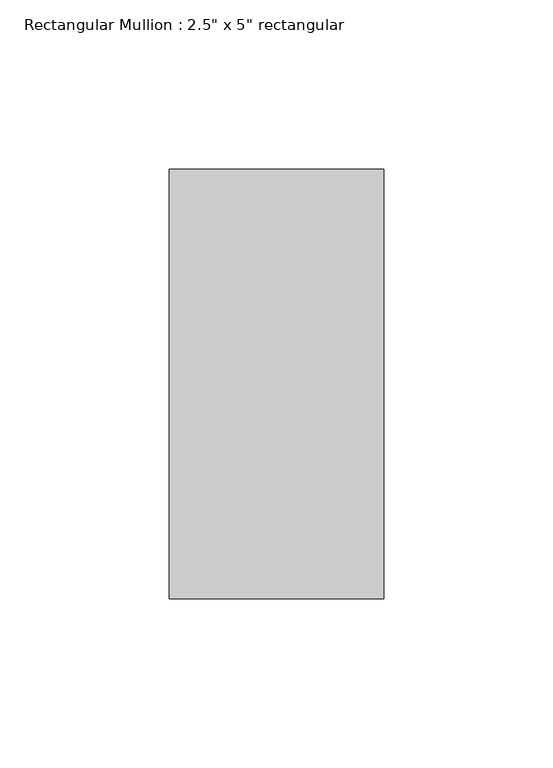
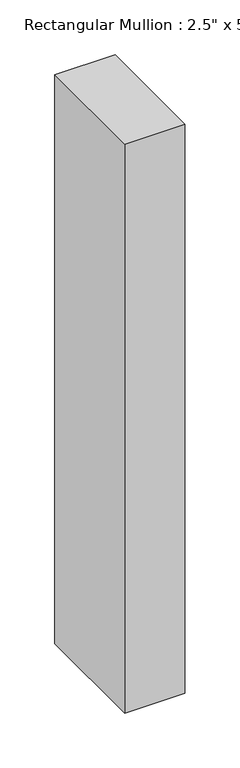
"""IFC4 building model written with IfcOpenShell, lengths in millimetres: member geometry."""

from ifc_helpers import new_model, si_unit, frame, origin, place, context, project, spatial, polyline, outline, extrude, source, transform, mapped, element, save


def member_7f909d8d(model_context):
    return source(origin(), model_context, "Body", "SweptSolid", [
        extrude(outline(polyline([(0.0, 63.5), (0.0, -63.5), (-63.5, -63.5), (-63.5, 63.5), (0.0, 63.5)])), frame((0.0, 0.0, -632.8833333), z_axis=(0.0, 0.0, 1.0), x_axis=(1.0, 0.0, 0.0)), (0.0, 0.0, 1.0), 632.8833333),
    ])


if __name__ == "__main__":
    model = new_model("IFC4")
    model_context = context("Model", 3, world=origin())
    ifc_project = project(units=[si_unit("LENGTHUNIT", "METRE", prefix="MILLI")], contexts=[model_context])
    site = spatial("IfcSite", under=ifc_project)
    building = spatial("IfcBuilding", under=site)
    placement = place(None, origin())
    member_shape = member_7f909d8d(model_context)
    element("IfcMember", 1, ObjectType="Rectangular Mullion : 2.5\" x 5\" rectangular", at=placement, inside=building, context=model_context, shape_type="MappedRepresentation", body=[
        mapped(member_shape, transform((0.0, 0.0, 0.0), x_axis=(1.0, 0.0, 0.0), y_axis=(0.0, 1.0, 0.0), z_axis=(0.0, 0.0, 1.0))),
    ])
    save(model, "model.ifc")

# Revit data of these elements
# Type "Rectangular Mullion : 2.5\" x 5\" rectangular"
#   built-in parameter 1007304 = 0.416667 (stored number, unit not read)
#   built-in parameter 1007301 = 0.104167 (stored number, unit not read)
#   built-in parameter 1007300 = 0.104167 (stored number, unit not read)
# Element 1 (IfcMember, "Rectangular Mullion : 2.5\" x 5\" rectangular")
#   Materials on its faces: "Aluminum"
# Materials
#   "Aluminum": class "Metal", colour RGB 247 247 247, transparency 0, Description = "Aluminum 6061", Cost = 0
